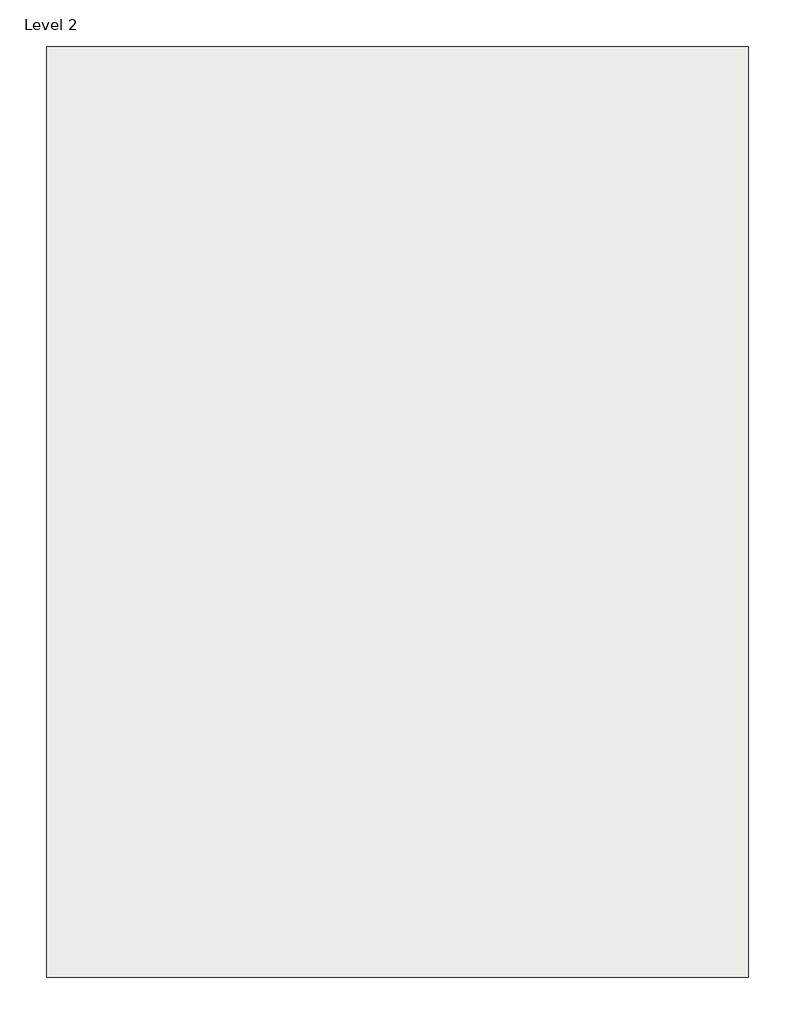
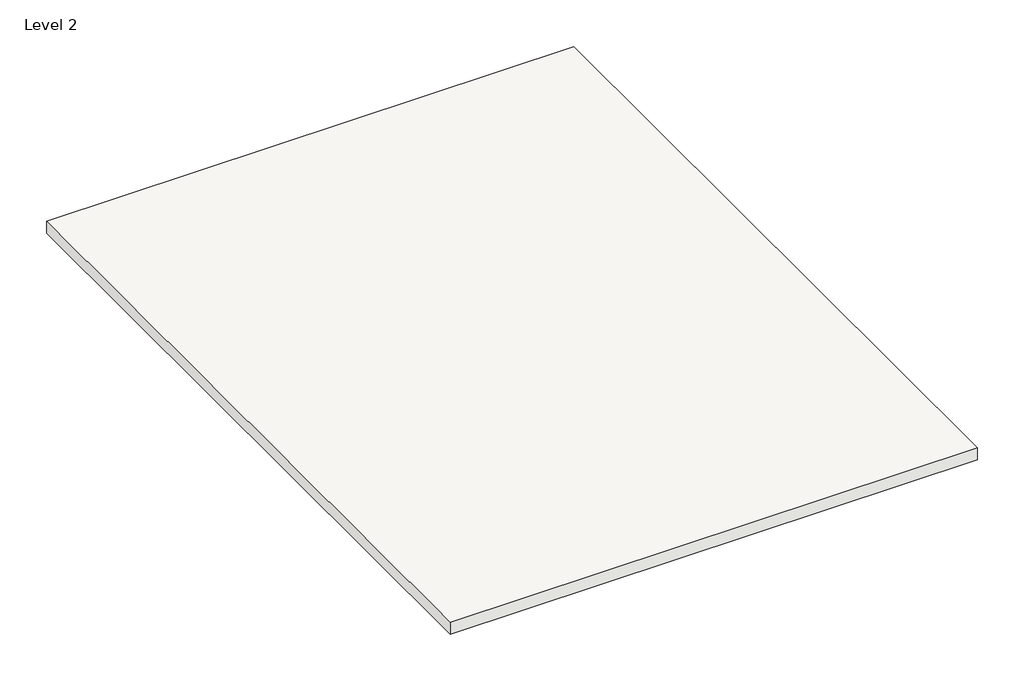
# One storey: 1 roof.
"""IFC4 building model written with IfcOpenShell, lengths in millimetres."""

from ifc_helpers import new_model, si_unit, frame, origin, place, context, project, spatial, polyline, outline, extrude, element, save

model = new_model("IFC4")

# Units and contexts
model_context = context("Model", 3, world=origin())
ifc_project = project(units=[si_unit("LENGTHUNIT", "METRE", prefix="MILLI")], contexts=[model_context])

# Site, building, storey
site = spatial("IfcSite", under=ifc_project)
building = spatial("IfcBuilding", under=site)
storey = spatial("IfcBuildingStorey", under=building, Name="Level 2", Elevation=3048.0)

# Roof
placement = place(None, origin())
element("IfcRoof", 1, ObjectType="Generic - 9\"", at=placement, inside=storey, context=model_context, shape_type="SweptSolid", body=[
    extrude(outline(polyline([(-10506.8128458, 14246.819734), (-1159.6128458, 14246.819734), (-1159.6128458, 1851.619734), (-10506.8128458, 1851.619734), (-10506.8128458, 14246.819734)])), frame((0.0, 0.0, 3048.0), z_axis=(0.0, 0.0, 1.0), x_axis=(1.0, 0.0, 0.0)), (0.0, 0.0, 1.0), 228.6),
])

save(model, "model.ifc")

# Revit data of these elements
# Type "Generic - 9\""
#   Assembly Code = "B1020"
#   Layers, outside or top first: 0' - 9" no material (function 1)
# Element 1 (IfcRoof, "Generic - 9\"")
#   built-in parameter 1001705 = 10.75 (stored number, unit not read)
#   built-in parameter 1001710 = 33615
#   Phase Created = New Construction
#   Materials on its faces: "Default Roof"
# Materials
#   "Default Roof": colour RGB 88 101 114, transparency 0
